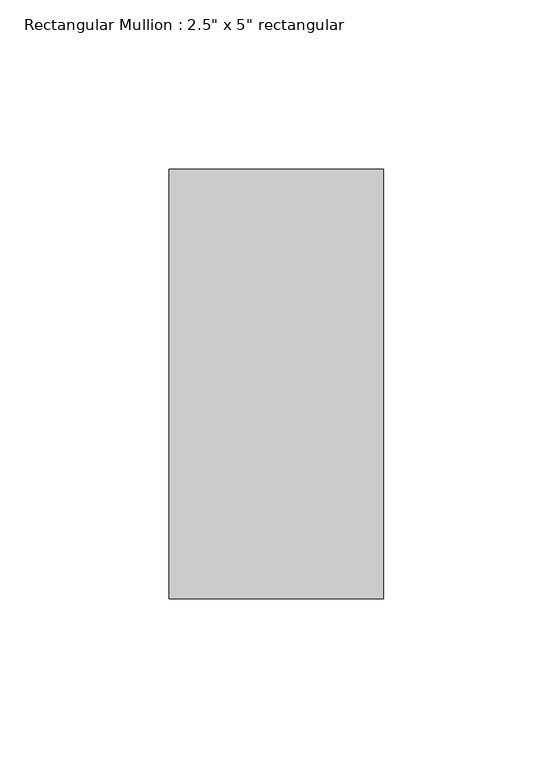
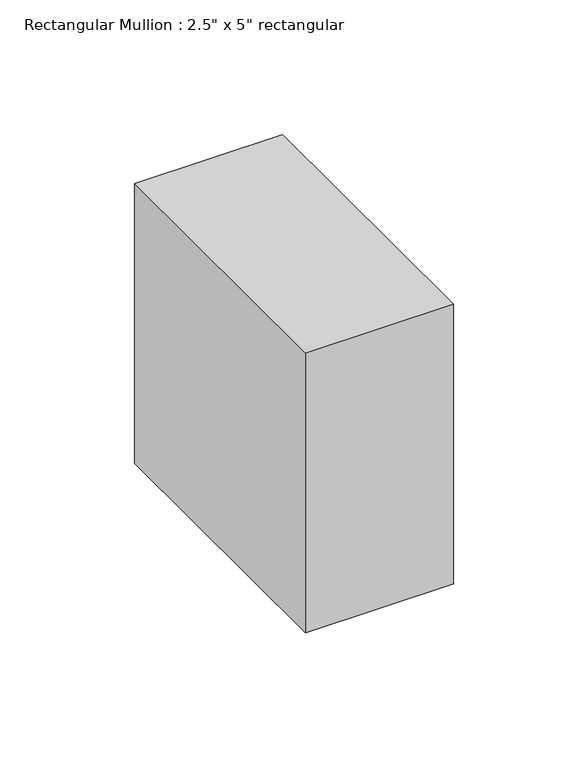
"""IFC4 building model written with IfcOpenShell, lengths in millimetres: member geometry."""

from ifc_helpers import new_model, si_unit, frame, origin, place, context, project, spatial, polyline, outline, extrude, source, transform, mapped, element, save


def member_7190e7de(model_context):
    return source(origin(), model_context, "Body", "SweptSolid", [
        extrude(outline(polyline([(31.75, 63.5), (31.75, -63.5), (-31.75, -63.5), (-31.75, 63.5), (31.75, 63.5)])), frame((0.0, 0.0, -127.0), z_axis=(0.0, 0.0, 1.0), x_axis=(1.0, 0.0, 0.0)), (0.0, 0.0, 1.0), 127.0),
    ])


if __name__ == "__main__":
    model = new_model("IFC4")
    model_context = context("Model", 3, world=origin())
    ifc_project = project(units=[si_unit("LENGTHUNIT", "METRE", prefix="MILLI")], contexts=[model_context])
    site = spatial("IfcSite", under=ifc_project)
    building = spatial("IfcBuilding", under=site)
    placement = place(None, origin())
    member_shape = member_7190e7de(model_context)
    element("IfcMember", 1, ObjectType="Rectangular Mullion : 2.5\" x 5\" rectangular", at=placement, inside=building, context=model_context, shape_type="MappedRepresentation", body=[
        mapped(member_shape, transform((0.0, 0.0, 0.0), x_axis=(1.0, 0.0, 0.0), y_axis=(0.0, 1.0, 0.0), z_axis=(0.0, 0.0, 1.0))),
    ])
    save(model, "model.ifc")

# Revit data of these elements
# Type "Rectangular Mullion : 2.5\" x 5\" rectangular"
#   built-in parameter 1007304 = 0.416667 (stored number, unit not read)
#   built-in parameter 1007301 = 0.104167 (stored number, unit not read)
#   built-in parameter 1007300 = 0.104167 (stored number, unit not read)
# Element 1 (IfcMember, "Rectangular Mullion : 2.5\" x 5\" rectangular")
#   Materials on its faces: "Aluminum"
# Materials
#   "Aluminum": class "Metal", colour RGB 247 247 247, transparency 0, Description = "Aluminum 6061", Cost = 0
